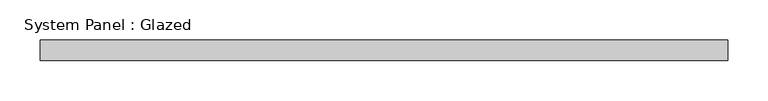
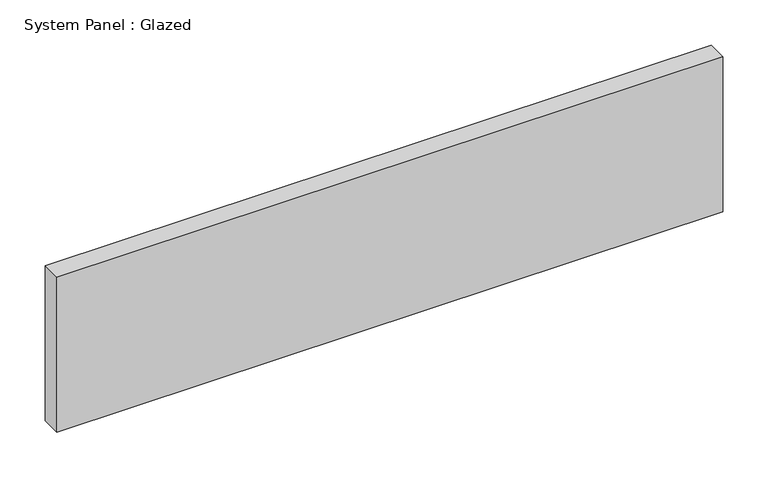
"""IFC4 building model written with IfcOpenShell, lengths in millimetres: plate geometry, System Panel : Glazed."""

from ifc_helpers import new_model, si_unit, origin, origin_with_axes, place, context, project, spatial, polyline, outline, extrude, source, transform, mapped, element, save


def system_panel_glazed_fbb6c980(model_context):
    return source(origin(), model_context, "Body", "SweptSolid", [
        extrude(outline(polyline([(425.45, 19.05), (-425.45, 19.05), (-425.45, 44.45), (425.45, 44.45), (425.45, 19.05)])), origin_with_axes(), (0.0, 0.0, 1.0), 209.55),
    ])


if __name__ == "__main__":
    model = new_model("IFC4")
    model_context = context("Model", 3, world=origin())
    ifc_project = project(units=[si_unit("LENGTHUNIT", "METRE", prefix="MILLI")], contexts=[model_context])
    site = spatial("IfcSite", under=ifc_project)
    building = spatial("IfcBuilding", under=site)
    placement = place(None, origin())
    system_panel_glazed_shape = system_panel_glazed_fbb6c980(model_context)
    element("IfcPlate", 1, ObjectType="System Panel : Glazed", at=placement, inside=building, context=model_context, shape_type="MappedRepresentation", body=[
        mapped(system_panel_glazed_shape, transform((0.0, 0.0, 0.0), x_axis=(1.0, 0.0, 0.0), y_axis=(0.0, 1.0, 0.0), z_axis=(0.0, 0.0, 1.0))),
    ])
    save(model, "model.ifc")

# Revit data of these elements
# Type "System Panel : Glazed"
#   Construction Type Id = "GSP4R"
#   Analytic Construction = "1/8 in Pilkington single glazing"
#   Visual Light Transmittance = 0.9
#   Solar Heat Gain Coefficient = 0.86
#   Heat Transfer Coefficient (U) = 6.7069 W/(m²·K)
# Element 1 (IfcPlate, "System Panel : Glazed")
#   Materials on its faces: "Glass"
# Materials
#   "Glass": class "Glass", colour RGB 0 128 192, transparency 0.75, Description = "Soda Lime Glass", Cost = 0
